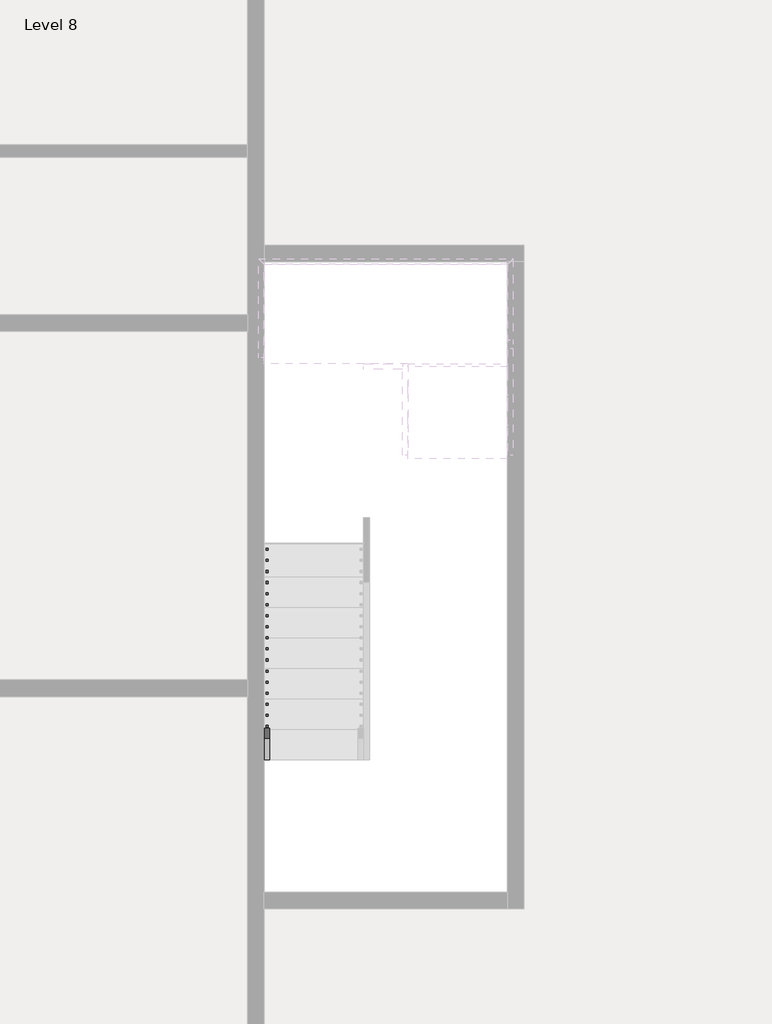
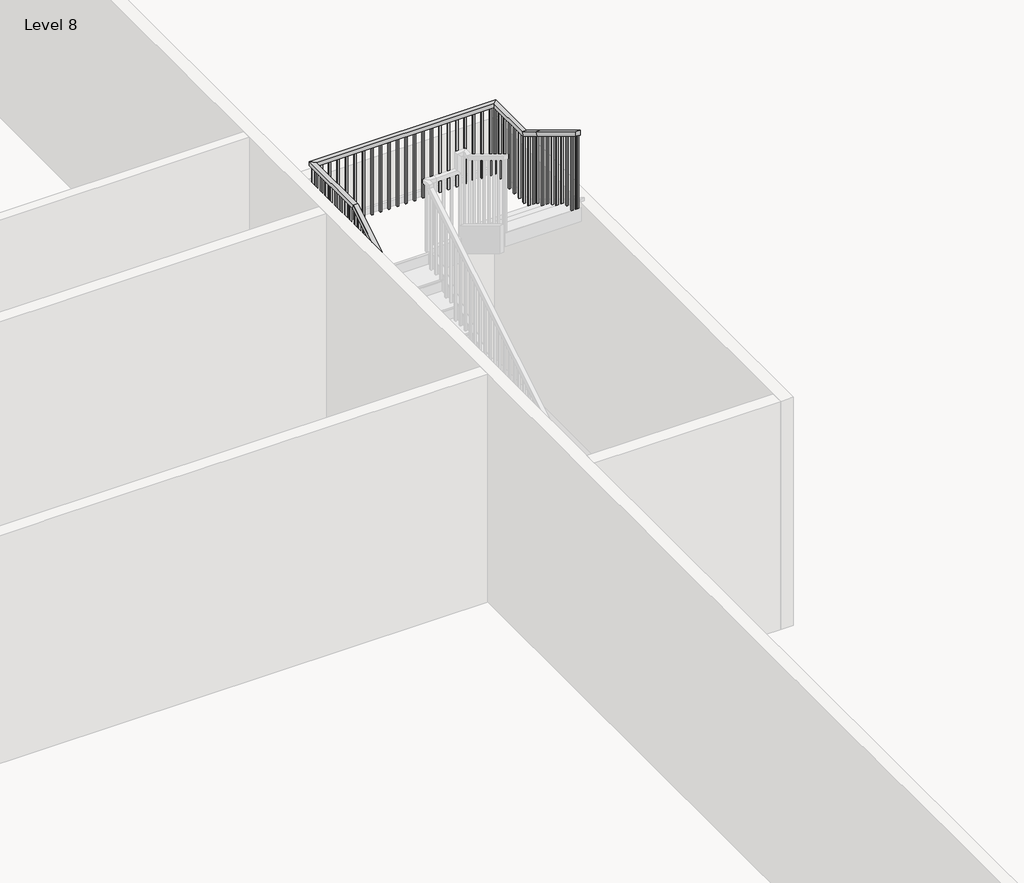
# One storey, part 6 of 8: 1 railing.
"""IFC4 building model written with IfcOpenShell, lengths in millimetres."""

from ifc_helpers import new_model, si_unit, frame, origin, place, context, project, spatial, polyline, outline, extrude, faceted_brep, element, save

model = new_model("IFC4")

# Units and contexts
model_context = context("Model", 3, world=origin())
ifc_project = project(units=[si_unit("LENGTHUNIT", "METRE", prefix="MILLI")], contexts=[model_context])

# Site, building, storey
site = spatial("IfcSite", under=ifc_project)
building = spatial("IfcBuilding", under=site)
storey = spatial("IfcBuildingStorey", under=building, Name="Level 8", Elevation=46570.6172466)

# Railing
placement = place(None, origin())
element("IfcRailing", 1, ObjectType="Handrail - Rectangular", at=placement, inside=storey, context=model_context, shape_type="SolidModel", body=[
    faceted_brep([(-3617.4415084, -23154.3851539, 47654.3505799), (-3617.4415084, -23154.3851539, 47594.9491197), (-3566.6415084, -23154.3851539, 47594.9491197), (-3566.6415084, -23154.3851539, 47654.3505799), (-3617.4415084, -19522.1851539, 49855.6839133), (-3617.4415084, -19507.9927445, 49804.8839133), (-3566.6415084, -19507.9927445, 49804.8839133), (-3566.6415084, -19522.1851539, 49855.6839133), (-3617.4415084, -18607.7851539, 49855.6839133), (-3617.4415084, -18607.7851539, 49804.8839133), (-3566.6415084, -18658.5851539, 49804.8839133), (-3566.6415084, -18658.5851539, 49855.6839133), (-1382.2415084, -18607.7851539, 49855.6839133), (-1382.2415084, -18607.7851539, 49804.8839133), (-1433.0415084, -18658.5851539, 49804.8839133), (-1433.0415084, -18658.5851539, 49855.6839133), (-1382.2415084, -19242.7851539, 49855.6839133), (-1382.2415084, -19256.9775633, 49804.8839133), (-1433.0415084, -19256.9775633, 49804.8839133), (-1433.0415084, -19242.7851539, 49855.6839133), (-1382.2415084, -19522.1851539, 50025.0172466), (-1382.2415084, -19548.5148811, 49981.5731968), (-1433.0415084, -19548.5148811, 49981.5731968), (-1433.0415084, -19522.1851539, 50025.0172466), (-1382.2415084, -20360.3851539, 50533.0172466), (-1433.0415084, -20360.3851539, 50533.0172466), (-1433.0415084, -20360.3851539, 50473.6157863), (-1382.2415084, -20360.3851539, 50473.6157863)], [[[0, 1, 2, 3]], [[1, 0, 4, 5]], [[2, 1, 5, 6]], [[3, 2, 6, 7]], [[0, 3, 7, 4]], [[5, 4, 8, 9]], [[6, 5, 9, 10]], [[7, 6, 10, 11]], [[4, 7, 11, 8]], [[9, 8, 12, 13]], [[10, 9, 13, 14]], [[11, 10, 14, 15]], [[8, 11, 15, 12]], [[13, 12, 16, 17]], [[14, 13, 17, 18]], [[15, 14, 18, 19]], [[12, 15, 19, 16]], [[17, 16, 20, 21]], [[18, 17, 21, 22]], [[19, 18, 22, 23]], [[16, 19, 23, 20]], [[24, 25, 26, 27]], [[21, 20, 24, 27]], [[22, 21, 27, 26]], [[23, 22, 26, 25]], [[20, 23, 25, 24]]]),
    extrude(outline(polyline([(-20325.4601539, 50452.4491197), (-20325.4601539, 49449.2839133), (-20344.5101539, 49449.2839133), (-20344.5101539, 50463.9945742), (-20325.4601539, 50452.4491197)])), frame((-1417.1665084, 0.0, 0.0), z_axis=(1.0, 0.0, 0.0), x_axis=(0.0, 1.0, 0.0)), (0.0, 0.0, 1.0), 19.05),
    extrude(outline(polyline([(-20223.8601539, 50390.8733621), (-20223.8601539, 49449.2839133), (-20242.9101539, 49449.2839133), (-20242.9101539, 50402.4188166), (-20223.8601539, 50390.8733621)])), frame((-1417.1665084, 0.0, 0.0), z_axis=(1.0, 0.0, 0.0), x_axis=(0.0, 1.0, 0.0)), (0.0, 0.0, 1.0), 19.05),
    extrude(outline(polyline([(-20122.2601539, 50329.2976045), (-20122.2601539, 49449.2839133), (-20141.3101539, 49449.2839133), (-20141.3101539, 50340.8430591), (-20122.2601539, 50329.2976045)])), frame((-1417.1665084, 0.0, 0.0), z_axis=(1.0, 0.0, 0.0), x_axis=(0.0, 1.0, 0.0)), (0.0, 0.0, 1.0), 19.05),
    extrude(outline(polyline([(-20020.6601539, 50267.721847), (-20020.6601539, 49279.9505799), (-20039.7101539, 49279.9505799), (-20039.7101539, 50279.2673015), (-20020.6601539, 50267.721847)])), frame((-1417.1665084, 0.0, 0.0), z_axis=(1.0, 0.0, 0.0), x_axis=(0.0, 1.0, 0.0)), (0.0, 0.0, 1.0), 19.05),
    extrude(outline(polyline([(-19919.0601539, 50206.1460894), (-19919.0601539, 49279.9505799), (-19938.1101539, 49279.9505799), (-19938.1101539, 50217.6915439), (-19919.0601539, 50206.1460894)])), frame((-1417.1665084, 0.0, 0.0), z_axis=(1.0, 0.0, 0.0), x_axis=(0.0, 1.0, 0.0)), (0.0, 0.0, 1.0), 19.05),
    extrude(outline(polyline([(-19817.4601539, 50144.5703318), (-19817.4601539, 49279.9505799), (-19836.5101539, 49279.9505799), (-19836.5101539, 50156.1157863), (-19817.4601539, 50144.5703318)])), frame((-1417.1665084, 0.0, 0.0), z_axis=(1.0, 0.0, 0.0), x_axis=(0.0, 1.0, 0.0)), (0.0, 0.0, 1.0), 19.05),
    extrude(outline(polyline([(-19715.8601539, 50082.9945742), (-19715.8601539, 49110.6172466), (-19734.9101539, 49110.6172466), (-19734.9101539, 50094.5400288), (-19715.8601539, 50082.9945742)])), frame((-1417.1665084, 0.0, 0.0), z_axis=(1.0, 0.0, 0.0), x_axis=(0.0, 1.0, 0.0)), (0.0, 0.0, 1.0), 19.05),
    extrude(outline(polyline([(-19614.2601539, 50021.4188166), (-19614.2601539, 49110.6172466), (-19633.3101539, 49110.6172466), (-19633.3101539, 50032.9642712), (-19614.2601539, 50021.4188166)])), frame((-1417.1665084, 0.0, 0.0), z_axis=(1.0, 0.0, 0.0), x_axis=(0.0, 1.0, 0.0)), (0.0, 0.0, 1.0), 19.05),
    extrude(outline(polyline([(-19436.4601539, 49913.6612409), (-19436.4601539, 48941.2839133), (-19455.5101539, 48941.2839133), (-19455.5101539, 49925.2066954), (-19436.4601539, 49913.6612409)])), frame((-1417.1665084, 0.0, 0.0), z_axis=(1.0, 0.0, 0.0), x_axis=(0.0, 1.0, 0.0)), (0.0, 0.0, 1.0), 19.05),
    extrude(outline(polyline([(-19334.8601539, 49852.0854833), (-19334.8601539, 48941.2839133), (-19353.9101539, 48941.2839133), (-19353.9101539, 49863.6309379), (-19334.8601539, 49852.0854833)])), frame((-1417.1665084, 0.0, 0.0), z_axis=(1.0, 0.0, 0.0), x_axis=(0.0, 1.0, 0.0)), (0.0, 0.0, 1.0), 19.05),
    extrude(outline(polyline([(-1398.1165084, -19233.2601539), (-1398.1165084, -19252.3101539), (-1417.1665084, -19252.3101539), (-1417.1665084, -19233.2601539), (-1398.1165084, -19233.2601539)])), frame((0.0, 0.0, 48941.2839133), z_axis=(0.0, 0.0, 1.0), x_axis=(1.0, 0.0, 0.0)), (0.0, 0.0, 1.0), 863.6),
    extrude(outline(polyline([(-1398.1165084, -19131.6601539), (-1398.1165084, -19150.7101539), (-1417.1665084, -19150.7101539), (-1417.1665084, -19131.6601539), (-1398.1165084, -19131.6601539)])), frame((0.0, 0.0, 48941.2839133), z_axis=(0.0, 0.0, 1.0), x_axis=(1.0, 0.0, 0.0)), (0.0, 0.0, 1.0), 863.6),
    extrude(outline(polyline([(-1398.1165084, -19030.0601539), (-1398.1165084, -19049.1101539), (-1417.1665084, -19049.1101539), (-1417.1665084, -19030.0601539), (-1398.1165084, -19030.0601539)])), frame((0.0, 0.0, 48941.2839133), z_axis=(0.0, 0.0, 1.0), x_axis=(1.0, 0.0, 0.0)), (0.0, 0.0, 1.0), 863.6),
    extrude(outline(polyline([(-1398.1165084, -18928.4601539), (-1398.1165084, -18947.5101539), (-1417.1665084, -18947.5101539), (-1417.1665084, -18928.4601539), (-1398.1165084, -18928.4601539)])), frame((0.0, 0.0, 48941.2839133), z_axis=(0.0, 0.0, 1.0), x_axis=(1.0, 0.0, 0.0)), (0.0, 0.0, 1.0), 863.6),
    extrude(outline(polyline([(-1398.1165084, -18826.8601539), (-1398.1165084, -18845.9101539), (-1417.1665084, -18845.9101539), (-1417.1665084, -18826.8601539), (-1398.1165084, -18826.8601539)])), frame((0.0, 0.0, 48941.2839133), z_axis=(0.0, 0.0, 1.0), x_axis=(1.0, 0.0, 0.0)), (0.0, 0.0, 1.0), 863.6),
    extrude(outline(polyline([(-1398.1165084, -18725.2601539), (-1398.1165084, -18744.3101539), (-1417.1665084, -18744.3101539), (-1417.1665084, -18725.2601539), (-1398.1165084, -18725.2601539)])), frame((0.0, 0.0, 48941.2839133), z_axis=(0.0, 0.0, 1.0), x_axis=(1.0, 0.0, 0.0)), (0.0, 0.0, 1.0), 863.6),
    extrude(outline(polyline([(-1467.9665084, -18623.6601539), (-1448.9165084, -18623.6601539), (-1448.9165084, -18642.7101539), (-1467.9665084, -18642.7101539), (-1467.9665084, -18623.6601539)])), frame((0.0, 0.0, 48941.2839133), z_axis=(0.0, 0.0, 1.0), x_axis=(1.0, 0.0, 0.0)), (0.0, 0.0, 1.0), 863.6),
    extrude(outline(polyline([(-1569.5665084, -18623.6601539), (-1550.5165084, -18623.6601539), (-1550.5165084, -18642.7101539), (-1569.5665084, -18642.7101539), (-1569.5665084, -18623.6601539)])), frame((0.0, 0.0, 48941.2839133), z_axis=(0.0, 0.0, 1.0), x_axis=(1.0, 0.0, 0.0)), (0.0, 0.0, 1.0), 863.6),
    extrude(outline(polyline([(-1671.1665084, -18623.6601539), (-1652.1165084, -18623.6601539), (-1652.1165084, -18642.7101539), (-1671.1665084, -18642.7101539), (-1671.1665084, -18623.6601539)])), frame((0.0, 0.0, 48941.2839133), z_axis=(0.0, 0.0, 1.0), x_axis=(1.0, 0.0, 0.0)), (0.0, 0.0, 1.0), 863.6),
    extrude(outline(polyline([(-1772.7665084, -18623.6601539), (-1753.7165084, -18623.6601539), (-1753.7165084, -18642.7101539), (-1772.7665084, -18642.7101539), (-1772.7665084, -18623.6601539)])), frame((0.0, 0.0, 48941.2839133), z_axis=(0.0, 0.0, 1.0), x_axis=(1.0, 0.0, 0.0)), (0.0, 0.0, 1.0), 863.6),
    extrude(outline(polyline([(-1874.3665084, -18623.6601539), (-1855.3165084, -18623.6601539), (-1855.3165084, -18642.7101539), (-1874.3665084, -18642.7101539), (-1874.3665084, -18623.6601539)])), frame((0.0, 0.0, 48941.2839133), z_axis=(0.0, 0.0, 1.0), x_axis=(1.0, 0.0, 0.0)), (0.0, 0.0, 1.0), 863.6),
    extrude(outline(polyline([(-1975.9665084, -18623.6601539), (-1956.9165084, -18623.6601539), (-1956.9165084, -18642.7101539), (-1975.9665084, -18642.7101539), (-1975.9665084, -18623.6601539)])), frame((0.0, 0.0, 48941.2839133), z_axis=(0.0, 0.0, 1.0), x_axis=(1.0, 0.0, 0.0)), (0.0, 0.0, 1.0), 863.6),
    extrude(outline(polyline([(-2077.5665084, -18623.6601539), (-2058.5165084, -18623.6601539), (-2058.5165084, -18642.7101539), (-2077.5665084, -18642.7101539), (-2077.5665084, -18623.6601539)])), frame((0.0, 0.0, 48941.2839133), z_axis=(0.0, 0.0, 1.0), x_axis=(1.0, 0.0, 0.0)), (0.0, 0.0, 1.0), 863.6),
    extrude(outline(polyline([(-2179.1665084, -18623.6601539), (-2160.1165084, -18623.6601539), (-2160.1165084, -18642.7101539), (-2179.1665084, -18642.7101539), (-2179.1665084, -18623.6601539)])), frame((0.0, 0.0, 48941.2839133), z_axis=(0.0, 0.0, 1.0), x_axis=(1.0, 0.0, 0.0)), (0.0, 0.0, 1.0), 863.6),
    extrude(outline(polyline([(-2280.7665084, -18623.6601539), (-2261.7165084, -18623.6601539), (-2261.7165084, -18642.7101539), (-2280.7665084, -18642.7101539), (-2280.7665084, -18623.6601539)])), frame((0.0, 0.0, 48941.2839133), z_axis=(0.0, 0.0, 1.0), x_axis=(1.0, 0.0, 0.0)), (0.0, 0.0, 1.0), 863.6),
    extrude(outline(polyline([(-2382.3665084, -18623.6601539), (-2363.3165084, -18623.6601539), (-2363.3165084, -18642.7101539), (-2382.3665084, -18642.7101539), (-2382.3665084, -18623.6601539)])), frame((0.0, 0.0, 48941.2839133), z_axis=(0.0, 0.0, 1.0), x_axis=(1.0, 0.0, 0.0)), (0.0, 0.0, 1.0), 863.6),
    extrude(outline(polyline([(-2483.9665084, -18623.6601539), (-2464.9165084, -18623.6601539), (-2464.9165084, -18642.7101539), (-2483.9665084, -18642.7101539), (-2483.9665084, -18623.6601539)])), frame((0.0, 0.0, 48941.2839133), z_axis=(0.0, 0.0, 1.0), x_axis=(1.0, 0.0, 0.0)), (0.0, 0.0, 1.0), 863.6),
    extrude(outline(polyline([(-2585.5665084, -18623.6601539), (-2566.5165084, -18623.6601539), (-2566.5165084, -18642.7101539), (-2585.5665084, -18642.7101539), (-2585.5665084, -18623.6601539)])), frame((0.0, 0.0, 48941.2839133), z_axis=(0.0, 0.0, 1.0), x_axis=(1.0, 0.0, 0.0)), (0.0, 0.0, 1.0), 863.6),
    extrude(outline(polyline([(-2687.1665084, -18623.6601539), (-2668.1165084, -18623.6601539), (-2668.1165084, -18642.7101539), (-2687.1665084, -18642.7101539), (-2687.1665084, -18623.6601539)])), frame((0.0, 0.0, 48941.2839133), z_axis=(0.0, 0.0, 1.0), x_axis=(1.0, 0.0, 0.0)), (0.0, 0.0, 1.0), 863.6),
    extrude(outline(polyline([(-2788.7665084, -18623.6601539), (-2769.7165084, -18623.6601539), (-2769.7165084, -18642.7101539), (-2788.7665084, -18642.7101539), (-2788.7665084, -18623.6601539)])), frame((0.0, 0.0, 48941.2839133), z_axis=(0.0, 0.0, 1.0), x_axis=(1.0, 0.0, 0.0)), (0.0, 0.0, 1.0), 863.6),
    extrude(outline(polyline([(-2890.3665084, -18623.6601539), (-2871.3165084, -18623.6601539), (-2871.3165084, -18642.7101539), (-2890.3665084, -18642.7101539), (-2890.3665084, -18623.6601539)])), frame((0.0, 0.0, 48941.2839133), z_axis=(0.0, 0.0, 1.0), x_axis=(1.0, 0.0, 0.0)), (0.0, 0.0, 1.0), 863.6),
    extrude(outline(polyline([(-2991.9665084, -18623.6601539), (-2972.9165084, -18623.6601539), (-2972.9165084, -18642.7101539), (-2991.9665084, -18642.7101539), (-2991.9665084, -18623.6601539)])), frame((0.0, 0.0, 48941.2839133), z_axis=(0.0, 0.0, 1.0), x_axis=(1.0, 0.0, 0.0)), (0.0, 0.0, 1.0), 863.6),
    extrude(outline(polyline([(-3093.5665084, -18623.6601539), (-3074.5165084, -18623.6601539), (-3074.5165084, -18642.7101539), (-3093.5665084, -18642.7101539), (-3093.5665084, -18623.6601539)])), frame((0.0, 0.0, 48941.2839133), z_axis=(0.0, 0.0, 1.0), x_axis=(1.0, 0.0, 0.0)), (0.0, 0.0, 1.0), 863.6),
    extrude(outline(polyline([(-3195.1665084, -18623.6601539), (-3176.1165084, -18623.6601539), (-3176.1165084, -18642.7101539), (-3195.1665084, -18642.7101539), (-3195.1665084, -18623.6601539)])), frame((0.0, 0.0, 48941.2839133), z_axis=(0.0, 0.0, 1.0), x_axis=(1.0, 0.0, 0.0)), (0.0, 0.0, 1.0), 863.6),
    extrude(outline(polyline([(-3296.7665084, -18623.6601539), (-3277.7165084, -18623.6601539), (-3277.7165084, -18642.7101539), (-3296.7665084, -18642.7101539), (-3296.7665084, -18623.6601539)])), frame((0.0, 0.0, 48941.2839133), z_axis=(0.0, 0.0, 1.0), x_axis=(1.0, 0.0, 0.0)), (0.0, 0.0, 1.0), 863.6),
    extrude(outline(polyline([(-3398.3665084, -18623.6601539), (-3379.3165084, -18623.6601539), (-3379.3165084, -18642.7101539), (-3398.3665084, -18642.7101539), (-3398.3665084, -18623.6601539)])), frame((0.0, 0.0, 48941.2839133), z_axis=(0.0, 0.0, 1.0), x_axis=(1.0, 0.0, 0.0)), (0.0, 0.0, 1.0), 863.6),
    extrude(outline(polyline([(-3499.9665084, -18623.6601539), (-3480.9165084, -18623.6601539), (-3480.9165084, -18642.7101539), (-3499.9665084, -18642.7101539), (-3499.9665084, -18623.6601539)])), frame((0.0, 0.0, 48941.2839133), z_axis=(0.0, 0.0, 1.0), x_axis=(1.0, 0.0, 0.0)), (0.0, 0.0, 1.0), 863.6),
    extrude(outline(polyline([(-3601.5665084, -18718.9101539), (-3601.5665084, -18699.8601539), (-3582.5165084, -18699.8601539), (-3582.5165084, -18718.9101539), (-3601.5665084, -18718.9101539)])), frame((0.0, 0.0, 48941.2839133), z_axis=(0.0, 0.0, 1.0), x_axis=(1.0, 0.0, 0.0)), (0.0, 0.0, 1.0), 863.6),
    extrude(outline(polyline([(-3601.5665084, -18820.5101539), (-3601.5665084, -18801.4601539), (-3582.5165084, -18801.4601539), (-3582.5165084, -18820.5101539), (-3601.5665084, -18820.5101539)])), frame((0.0, 0.0, 48941.2839133), z_axis=(0.0, 0.0, 1.0), x_axis=(1.0, 0.0, 0.0)), (0.0, 0.0, 1.0), 863.6),
    extrude(outline(polyline([(-3601.5665084, -18922.1101539), (-3601.5665084, -18903.0601539), (-3582.5165084, -18903.0601539), (-3582.5165084, -18922.1101539), (-3601.5665084, -18922.1101539)])), frame((0.0, 0.0, 48941.2839133), z_axis=(0.0, 0.0, 1.0), x_axis=(1.0, 0.0, 0.0)), (0.0, 0.0, 1.0), 863.6),
    extrude(outline(polyline([(-3601.5665084, -19023.7101539), (-3601.5665084, -19004.6601539), (-3582.5165084, -19004.6601539), (-3582.5165084, -19023.7101539), (-3601.5665084, -19023.7101539)])), frame((0.0, 0.0, 48941.2839133), z_axis=(0.0, 0.0, 1.0), x_axis=(1.0, 0.0, 0.0)), (0.0, 0.0, 1.0), 863.6),
    extrude(outline(polyline([(-3601.5665084, -19125.3101539), (-3601.5665084, -19106.2601539), (-3582.5165084, -19106.2601539), (-3582.5165084, -19125.3101539), (-3601.5665084, -19125.3101539)])), frame((0.0, 0.0, 48941.2839133), z_axis=(0.0, 0.0, 1.0), x_axis=(1.0, 0.0, 0.0)), (0.0, 0.0, 1.0), 863.6),
    extrude(outline(polyline([(-3601.5665084, -19226.9101539), (-3601.5665084, -19207.8601539), (-3582.5165084, -19207.8601539), (-3582.5165084, -19226.9101539), (-3601.5665084, -19226.9101539)])), frame((0.0, 0.0, 48941.2839133), z_axis=(0.0, 0.0, 1.0), x_axis=(1.0, 0.0, 0.0)), (0.0, 0.0, 1.0), 863.6),
    extrude(outline(polyline([(-3601.5665084, -19328.5101539), (-3601.5665084, -19309.4601539), (-3582.5165084, -19309.4601539), (-3582.5165084, -19328.5101539), (-3601.5665084, -19328.5101539)])), frame((0.0, 0.0, 48941.2839133), z_axis=(0.0, 0.0, 1.0), x_axis=(1.0, 0.0, 0.0)), (0.0, 0.0, 1.0), 863.6),
    extrude(outline(polyline([(-3601.5665084, -19430.1101539), (-3601.5665084, -19411.0601539), (-3582.5165084, -19411.0601539), (-3582.5165084, -19430.1101539), (-3601.5665084, -19430.1101539)])), frame((0.0, 0.0, 48941.2839133), z_axis=(0.0, 0.0, 1.0), x_axis=(1.0, 0.0, 0.0)), (0.0, 0.0, 1.0), 863.6),
    extrude(outline(polyline([(-19588.8601539, 49755.8733621), (-19588.8601539, 48771.9505799), (-19607.9101539, 48771.9505799), (-19607.9101539, 49744.3279076), (-19588.8601539, 49755.8733621)])), frame((-3601.5665084, 0.0, 0.0), z_axis=(1.0, 0.0, 0.0), x_axis=(0.0, 1.0, 0.0)), (0.0, 0.0, 1.0), 19.05),
    extrude(outline(polyline([(-19690.4601539, 49694.2976045), (-19690.4601539, 48771.9505799), (-19709.5101539, 48771.9505799), (-19709.5101539, 49682.75215), (-19690.4601539, 49694.2976045)])), frame((-3601.5665084, 0.0, 0.0), z_axis=(1.0, 0.0, 0.0), x_axis=(0.0, 1.0, 0.0)), (0.0, 0.0, 1.0), 19.05),
    extrude(outline(polyline([(-19792.0601539, 49632.721847), (-19792.0601539, 48771.9505799), (-19811.1101539, 48771.9505799), (-19811.1101539, 49621.1763924), (-19792.0601539, 49632.721847)])), frame((-3601.5665084, 0.0, 0.0), z_axis=(1.0, 0.0, 0.0), x_axis=(0.0, 1.0, 0.0)), (0.0, 0.0, 1.0), 19.05),
    extrude(outline(polyline([(-19893.6601539, 49571.1460894), (-19893.6601539, 48602.6172466), (-19912.7101539, 48602.6172466), (-19912.7101539, 49559.6006348), (-19893.6601539, 49571.1460894)])), frame((-3601.5665084, 0.0, 0.0), z_axis=(1.0, 0.0, 0.0), x_axis=(0.0, 1.0, 0.0)), (0.0, 0.0, 1.0), 19.05),
    extrude(outline(polyline([(-19995.2601539, 49509.5703318), (-19995.2601539, 48602.6172466), (-20014.3101539, 48602.6172466), (-20014.3101539, 49498.0248773), (-19995.2601539, 49509.5703318)])), frame((-3601.5665084, 0.0, 0.0), z_axis=(1.0, 0.0, 0.0), x_axis=(0.0, 1.0, 0.0)), (0.0, 0.0, 1.0), 19.05),
    extrude(outline(polyline([(-20096.8601539, 49447.9945742), (-20096.8601539, 48433.2839133), (-20115.9101539, 48433.2839133), (-20115.9101539, 49436.4491197), (-20096.8601539, 49447.9945742)])), frame((-3601.5665084, 0.0, 0.0), z_axis=(1.0, 0.0, 0.0), x_axis=(0.0, 1.0, 0.0)), (0.0, 0.0, 1.0), 19.05),
    extrude(outline(polyline([(-20198.4601539, 49386.4188166), (-20198.4601539, 48433.2839133), (-20217.5101539, 48433.2839133), (-20217.5101539, 49374.8733621), (-20198.4601539, 49386.4188166)])), frame((-3601.5665084, 0.0, 0.0), z_axis=(1.0, 0.0, 0.0), x_axis=(0.0, 1.0, 0.0)), (0.0, 0.0, 1.0), 19.05),
    extrude(outline(polyline([(-20300.0601539, 49324.8430591), (-20300.0601539, 48433.2839133), (-20319.1101539, 48433.2839133), (-20319.1101539, 49313.2976045), (-20300.0601539, 49324.8430591)])), frame((-3601.5665084, 0.0, 0.0), z_axis=(1.0, 0.0, 0.0), x_axis=(0.0, 1.0, 0.0)), (0.0, 0.0, 1.0), 19.05),
    extrude(outline(polyline([(-20401.6601539, 49263.2673015), (-20401.6601539, 48263.9505799), (-20420.7101539, 48263.9505799), (-20420.7101539, 49251.721847), (-20401.6601539, 49263.2673015)])), frame((-3601.5665084, 0.0, 0.0), z_axis=(1.0, 0.0, 0.0), x_axis=(0.0, 1.0, 0.0)), (0.0, 0.0, 1.0), 19.05),
    extrude(outline(polyline([(-20503.2601539, 49201.6915439), (-20503.2601539, 48263.9505799), (-20522.3101539, 48263.9505799), (-20522.3101539, 49190.1460894), (-20503.2601539, 49201.6915439)])), frame((-3601.5665084, 0.0, 0.0), z_axis=(1.0, 0.0, 0.0), x_axis=(0.0, 1.0, 0.0)), (0.0, 0.0, 1.0), 19.05),
    extrude(outline(polyline([(-20604.8601539, 49140.1157863), (-20604.8601539, 48263.9505799), (-20623.9101539, 48263.9505799), (-20623.9101539, 49128.5703318), (-20604.8601539, 49140.1157863)])), frame((-3601.5665084, 0.0, 0.0), z_axis=(1.0, 0.0, 0.0), x_axis=(0.0, 1.0, 0.0)), (0.0, 0.0, 1.0), 19.05),
    extrude(outline(polyline([(-20706.4601539, 49078.5400288), (-20706.4601539, 48094.6172466), (-20725.5101539, 48094.6172466), (-20725.5101539, 49066.9945742), (-20706.4601539, 49078.5400288)])), frame((-3601.5665084, 0.0, 0.0), z_axis=(1.0, 0.0, 0.0), x_axis=(0.0, 1.0, 0.0)), (0.0, 0.0, 1.0), 19.05),
    extrude(outline(polyline([(-20808.0601539, 49016.9642712), (-20808.0601539, 48094.6172466), (-20827.1101539, 48094.6172466), (-20827.1101539, 49005.4188166), (-20808.0601539, 49016.9642712)])), frame((-3601.5665084, 0.0, 0.0), z_axis=(1.0, 0.0, 0.0), x_axis=(0.0, 1.0, 0.0)), (0.0, 0.0, 1.0), 19.05),
    extrude(outline(polyline([(-20909.6601539, 48955.3885136), (-20909.6601539, 48094.6172466), (-20928.7101539, 48094.6172466), (-20928.7101539, 48943.8430591), (-20909.6601539, 48955.3885136)])), frame((-3601.5665084, 0.0, 0.0), z_axis=(1.0, 0.0, 0.0), x_axis=(0.0, 1.0, 0.0)), (0.0, 0.0, 1.0), 19.05),
    extrude(outline(polyline([(-21011.2601539, 48893.812756), (-21011.2601539, 47925.2839133), (-21030.3101539, 47925.2839133), (-21030.3101539, 48882.2673015), (-21011.2601539, 48893.812756)])), frame((-3601.5665084, 0.0, 0.0), z_axis=(1.0, 0.0, 0.0), x_axis=(0.0, 1.0, 0.0)), (0.0, 0.0, 1.0), 19.05),
    extrude(outline(polyline([(-21112.8601539, 48832.2369985), (-21112.8601539, 47925.2839133), (-21131.9101539, 47925.2839133), (-21131.9101539, 48820.6915439), (-21112.8601539, 48832.2369985)])), frame((-3601.5665084, 0.0, 0.0), z_axis=(1.0, 0.0, 0.0), x_axis=(0.0, 1.0, 0.0)), (0.0, 0.0, 1.0), 19.05),
    extrude(outline(polyline([(-21214.4601539, 48770.6612409), (-21214.4601539, 47755.9505799), (-21233.5101539, 47755.9505799), (-21233.5101539, 48759.1157863), (-21214.4601539, 48770.6612409)])), frame((-3601.5665084, 0.0, 0.0), z_axis=(1.0, 0.0, 0.0), x_axis=(0.0, 1.0, 0.0)), (0.0, 0.0, 1.0), 19.05),
    extrude(outline(polyline([(-21316.0601539, 48709.0854833), (-21316.0601539, 47755.9505799), (-21335.1101539, 47755.9505799), (-21335.1101539, 48697.5400288), (-21316.0601539, 48709.0854833)])), frame((-3601.5665084, 0.0, 0.0), z_axis=(1.0, 0.0, 0.0), x_axis=(0.0, 1.0, 0.0)), (0.0, 0.0, 1.0), 19.05),
    extrude(outline(polyline([(-21417.6601539, 48647.5097257), (-21417.6601539, 47755.9505799), (-21436.7101539, 47755.9505799), (-21436.7101539, 48635.9642712), (-21417.6601539, 48647.5097257)])), frame((-3601.5665084, 0.0, 0.0), z_axis=(1.0, 0.0, 0.0), x_axis=(0.0, 1.0, 0.0)), (0.0, 0.0, 1.0), 19.05),
    extrude(outline(polyline([(-21519.2601539, 48585.9339682), (-21519.2601539, 47586.6172466), (-21538.3101539, 47586.6172466), (-21538.3101539, 48574.3885136), (-21519.2601539, 48585.9339682)])), frame((-3601.5665084, 0.0, 0.0), z_axis=(1.0, 0.0, 0.0), x_axis=(0.0, 1.0, 0.0)), (0.0, 0.0, 1.0), 19.05),
    extrude(outline(polyline([(-21620.8601539, 48524.3582106), (-21620.8601539, 47586.6172466), (-21639.9101539, 47586.6172466), (-21639.9101539, 48512.812756), (-21620.8601539, 48524.3582106)])), frame((-3601.5665084, 0.0, 0.0), z_axis=(1.0, 0.0, 0.0), x_axis=(0.0, 1.0, 0.0)), (0.0, 0.0, 1.0), 19.05),
    extrude(outline(polyline([(-21722.4601539, 48462.782453), (-21722.4601539, 47586.6172466), (-21741.5101539, 47586.6172466), (-21741.5101539, 48451.2369985), (-21722.4601539, 48462.782453)])), frame((-3601.5665084, 0.0, 0.0), z_axis=(1.0, 0.0, 0.0), x_axis=(0.0, 1.0, 0.0)), (0.0, 0.0, 1.0), 19.05),
    extrude(outline(polyline([(-21824.0601539, 48401.2066954), (-21824.0601539, 47417.2839133), (-21843.1101539, 47417.2839133), (-21843.1101539, 48389.6612409), (-21824.0601539, 48401.2066954)])), frame((-3601.5665084, 0.0, 0.0), z_axis=(1.0, 0.0, 0.0), x_axis=(0.0, 1.0, 0.0)), (0.0, 0.0, 1.0), 19.05),
    extrude(outline(polyline([(-21925.6601539, 48339.6309379), (-21925.6601539, 47417.2839133), (-21944.7101539, 47417.2839133), (-21944.7101539, 48328.0854833), (-21925.6601539, 48339.6309379)])), frame((-3601.5665084, 0.0, 0.0), z_axis=(1.0, 0.0, 0.0), x_axis=(0.0, 1.0, 0.0)), (0.0, 0.0, 1.0), 19.05),
    extrude(outline(polyline([(-22027.2601539, 48278.0551803), (-22027.2601539, 47417.2839133), (-22046.3101539, 47417.2839133), (-22046.3101539, 48266.5097257), (-22027.2601539, 48278.0551803)])), frame((-3601.5665084, 0.0, 0.0), z_axis=(1.0, 0.0, 0.0), x_axis=(0.0, 1.0, 0.0)), (0.0, 0.0, 1.0), 19.05),
    extrude(outline(polyline([(-22128.8601539, 48216.4794227), (-22128.8601539, 47247.9505799), (-22147.9101539, 47247.9505799), (-22147.9101539, 48204.9339682), (-22128.8601539, 48216.4794227)])), frame((-3601.5665084, 0.0, 0.0), z_axis=(1.0, 0.0, 0.0), x_axis=(0.0, 1.0, 0.0)), (0.0, 0.0, 1.0), 19.05),
    extrude(outline(polyline([(-22230.4601539, 48154.9036651), (-22230.4601539, 47247.9505799), (-22249.5101539, 47247.9505799), (-22249.5101539, 48143.3582106), (-22230.4601539, 48154.9036651)])), frame((-3601.5665084, 0.0, 0.0), z_axis=(1.0, 0.0, 0.0), x_axis=(0.0, 1.0, 0.0)), (0.0, 0.0, 1.0), 19.05),
    extrude(outline(polyline([(-22332.0601539, 48093.3279076), (-22332.0601539, 47078.6172466), (-22351.1101539, 47078.6172466), (-22351.1101539, 48081.782453), (-22332.0601539, 48093.3279076)])), frame((-3601.5665084, 0.0, 0.0), z_axis=(1.0, 0.0, 0.0), x_axis=(0.0, 1.0, 0.0)), (0.0, 0.0, 1.0), 19.05),
    extrude(outline(polyline([(-22433.6601539, 48031.75215), (-22433.6601539, 47078.6172466), (-22452.7101539, 47078.6172466), (-22452.7101539, 48020.2066954), (-22433.6601539, 48031.75215)])), frame((-3601.5665084, 0.0, 0.0), z_axis=(1.0, 0.0, 0.0), x_axis=(0.0, 1.0, 0.0)), (0.0, 0.0, 1.0), 19.05),
    extrude(outline(polyline([(-22535.2601539, 47970.1763924), (-22535.2601539, 47078.6172466), (-22554.3101539, 47078.6172466), (-22554.3101539, 47958.6309379), (-22535.2601539, 47970.1763924)])), frame((-3601.5665084, 0.0, 0.0), z_axis=(1.0, 0.0, 0.0), x_axis=(0.0, 1.0, 0.0)), (0.0, 0.0, 1.0), 19.05),
    extrude(outline(polyline([(-22636.8601539, 47908.6006348), (-22636.8601539, 46909.2839133), (-22655.9101539, 46909.2839133), (-22655.9101539, 47897.0551803), (-22636.8601539, 47908.6006348)])), frame((-3601.5665084, 0.0, 0.0), z_axis=(1.0, 0.0, 0.0), x_axis=(0.0, 1.0, 0.0)), (0.0, 0.0, 1.0), 19.05),
    extrude(outline(polyline([(-22738.4601539, 47847.0248773), (-22738.4601539, 46909.2839133), (-22757.5101539, 46909.2839133), (-22757.5101539, 47835.4794227), (-22738.4601539, 47847.0248773)])), frame((-3601.5665084, 0.0, 0.0), z_axis=(1.0, 0.0, 0.0), x_axis=(0.0, 1.0, 0.0)), (0.0, 0.0, 1.0), 19.05),
    extrude(outline(polyline([(-22840.0601539, 47785.4491197), (-22840.0601539, 46909.2839133), (-22859.1101539, 46909.2839133), (-22859.1101539, 47773.9036651), (-22840.0601539, 47785.4491197)])), frame((-3601.5665084, 0.0, 0.0), z_axis=(1.0, 0.0, 0.0), x_axis=(0.0, 1.0, 0.0)), (0.0, 0.0, 1.0), 19.05),
    extrude(outline(polyline([(-22941.6601539, 47723.8733621), (-22941.6601539, 46739.9505799), (-22960.7101539, 46739.9505799), (-22960.7101539, 47712.3279076), (-22941.6601539, 47723.8733621)])), frame((-3601.5665084, 0.0, 0.0), z_axis=(1.0, 0.0, 0.0), x_axis=(0.0, 1.0, 0.0)), (0.0, 0.0, 1.0), 19.05),
    extrude(outline(polyline([(-23043.2601539, 47662.2976045), (-23043.2601539, 46739.9505799), (-23062.3101539, 46739.9505799), (-23062.3101539, 47650.75215), (-23043.2601539, 47662.2976045)])), frame((-3601.5665084, 0.0, 0.0), z_axis=(1.0, 0.0, 0.0), x_axis=(0.0, 1.0, 0.0)), (0.0, 0.0, 1.0), 19.05),
    extrude(outline(polyline([(-19512.6601539, 49959.8430591), (-19512.6601539, 48941.2839133), (-19531.7101539, 48941.2839133), (-19531.7101539, 49971.3885136), (-19512.6601539, 49959.8430591)])), frame((-1417.1665084, 0.0, 0.0), z_axis=(1.0, 0.0, 0.0), x_axis=(0.0, 1.0, 0.0)), (0.0, 0.0, 1.0), 19.05),
    extrude(outline(polyline([(-1417.1665084, -18623.6601539), (-1398.1165084, -18623.6601539), (-1398.1165084, -18642.7101539), (-1417.1665084, -18642.7101539), (-1417.1665084, -18623.6601539)])), frame((0.0, 0.0, 48941.2839133), z_axis=(0.0, 0.0, 1.0), x_axis=(1.0, 0.0, 0.0)), (0.0, 0.0, 1.0), 863.6),
    extrude(outline(polyline([(-3601.5665084, -18642.7101539), (-3601.5665084, -18623.6601539), (-3582.5165084, -18623.6601539), (-3582.5165084, -18642.7101539), (-3601.5665084, -18642.7101539)])), frame((0.0, 0.0, 48941.2839133), z_axis=(0.0, 0.0, 1.0), x_axis=(1.0, 0.0, 0.0)), (0.0, 0.0, 1.0), 863.6),
    extrude(outline(polyline([(-19512.6601539, 49802.0551803), (-19512.6601539, 48941.2839133), (-19531.7101539, 48941.2839133), (-19531.7101539, 49790.5097257), (-19512.6601539, 49802.0551803)])), frame((-3601.5665084, 0.0, 0.0), z_axis=(1.0, 0.0, 0.0), x_axis=(0.0, 1.0, 0.0)), (0.0, 0.0, 1.0), 19.05),
    extrude(outline(polyline([(-20341.3351539, 50462.0703318), (-20341.3351539, 49449.2839133), (-20360.3851539, 49449.2839133), (-20360.3851539, 50473.6157863), (-20341.3351539, 50462.0703318)])), frame((-1417.1665084, 0.0, 0.0), z_axis=(1.0, 0.0, 0.0), x_axis=(0.0, 1.0, 0.0)), (0.0, 0.0, 1.0), 19.05),
    extrude(outline(polyline([(-23135.3351539, 47606.4945742), (-23135.3351539, 46739.9505799), (-23154.3851539, 46739.9505799), (-23154.3851539, 47594.9491197), (-23135.3351539, 47606.4945742)])), frame((-3601.5665084, 0.0, 0.0), z_axis=(1.0, 0.0, 0.0), x_axis=(0.0, 1.0, 0.0)), (0.0, 0.0, 1.0), 19.05),
])

save(model, "model.ifc")

# Revit data of these elements
# Type "Handrail - Rectangular"
#   Assembly Code = "C2010400"
#   built-in parameter 1008612 = 0.0416667 (stored number, unit not read)
#   built-in parameter 1008611 = 0.0416667 (stored number, unit not read)
#   built-in parameter 1008609 = 0.333333 (stored number, unit not read)
#   built-in parameter 1008604 = 0.166667 (stored number, unit not read)
#   built-in parameter 1008603 = 0.166667 (stored number, unit not read)
#   Railing Height = 3' - 0"
#   built-in parameter 1008630 = 2
#   built-in parameter 1008610 = 2
#   built-in parameter 1008618 = Baluster - Square : 3/4"
# Element 1 (IfcRailing, "Handrail - Rectangular")
#   Phase Created = New Construction
